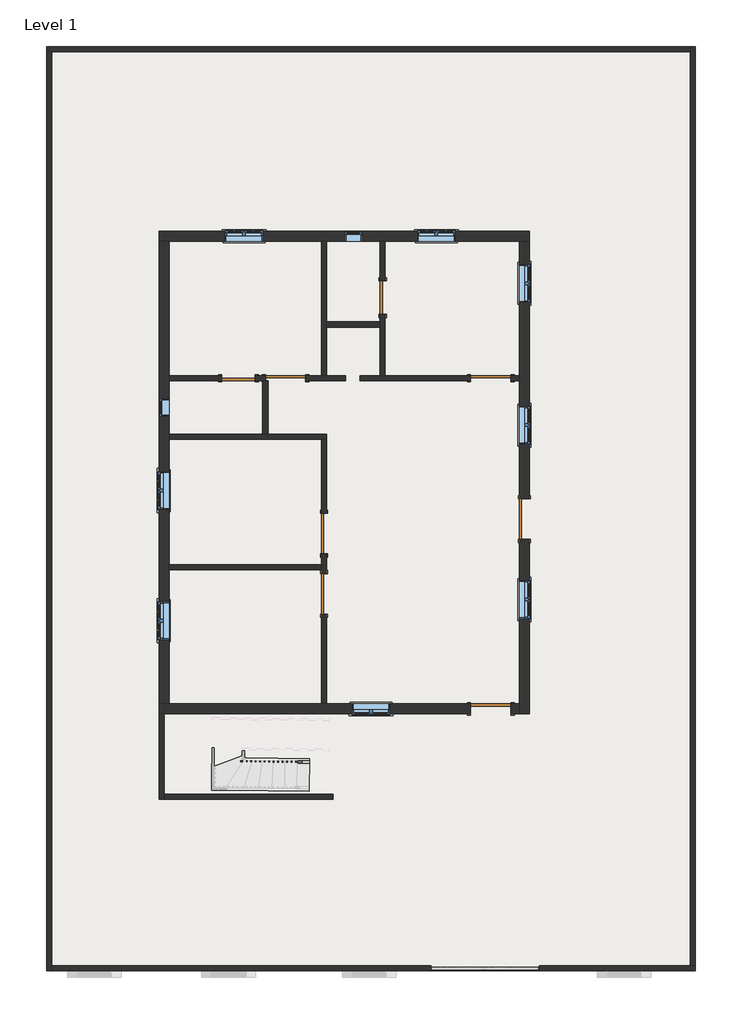
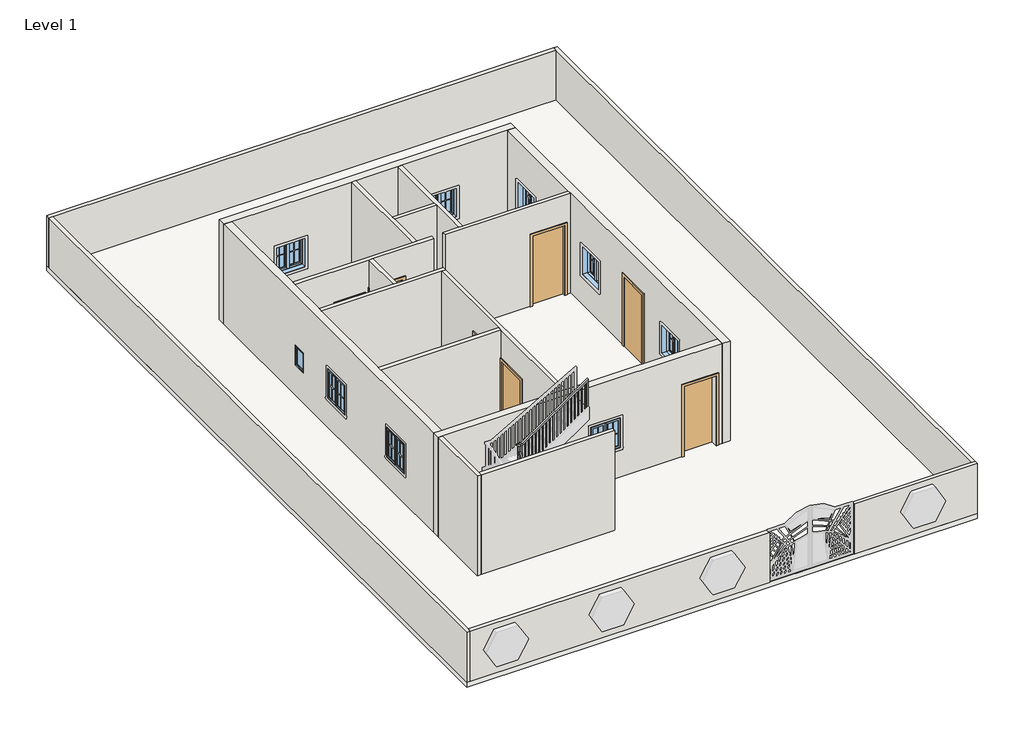
# One storey, part 1 of 2: 20 walls, 10 windows, 8 doors, 1 railing, 1 slab.
# Revit data of these elements (continued)
# Element 38 (IfcWindow, "Window-Casement-Double : 34\" x 36\"") (continued)
#   Interior Wall Closure = 0' - 2 1/4"
#   Frame Extension = 0' - 0 1/4"
#   Exterior Wall Closure = 0' - 1 1/4"
#   Interior Trim Visibility = yes
#   Exterior Trim Visibility = yes
#   Phase Created = New Construction
#   Materials on its faces: "Wood - Stained", "Glass", "Clad - White"
# Element 39 (IfcWindow, "Window-Casement-Double : 34\" x 36\"")
#   Mark = "9"
#   Window Inset = 0' - 0"
#   Interior Wall Closure = 0' - 2 1/4"
#   Frame Extension = 0' - 0 1/4"
#   Exterior Wall Closure = 0' - 1 1/4"
#   Interior Trim Visibility = yes
#   Exterior Trim Visibility = yes
#   Phase Created = New Construction
#   Materials on its faces: "Wood - Stained", "Glass", "Clad - White"
# Element 40 (IfcWindow, "Window-Casement-Double : 34\" x 36\"")
#   Mark = "10"
#   Window Inset = 0' - 0"
#   Interior Wall Closure = 0' - 2 1/4"
#   Frame Extension = 0' - 0 1/4"
#   Exterior Wall Closure = 0' - 1 1/4"
#   Interior Trim Visibility = yes
#   Exterior Trim Visibility = yes
#   Phase Created = New Construction
#   Materials on its faces: "Wood - Stained", "Glass", "Clad - White"
# Materials
#   "Door - Panel": class "Wood", colour RGB 210 159 95, transparency 0, Cost = 0
#   "Door - Frame": colour RGB 118 70 51, transparency 0, Cost = 0
#   "Glass": class "Glass", colour RGB 0 128 192, transparency 0.75, Description = "Soda Lime Glass", Cost = 0
#   "Sash": class "Wood", colour RGB 224 178 126, transparency 0, Cost = 0
#   "Wood - Stained": class "Wood", colour RGB 224 178 126, transparency 0, Cost = 0
#   "Clad - White": class "Wood", colour RGB 242 242 238, transparency 0, Cost = 0
#   "Default Floor": colour RGB 128 128 128, transparency 0, Cost = 0
#   "Cherry": class "Wood", colour RGB 226 177 128, transparency 0, Description = "Prunus Serotina", Cost = 0
#   "Default Wall": colour RGB 128 128 128, transparency 0, Cost = 0
#   "Carpet (1)": class "Carpet", colour RGB 124 80 67, transparency 0, Description = "Interior finish", Cost = 0
